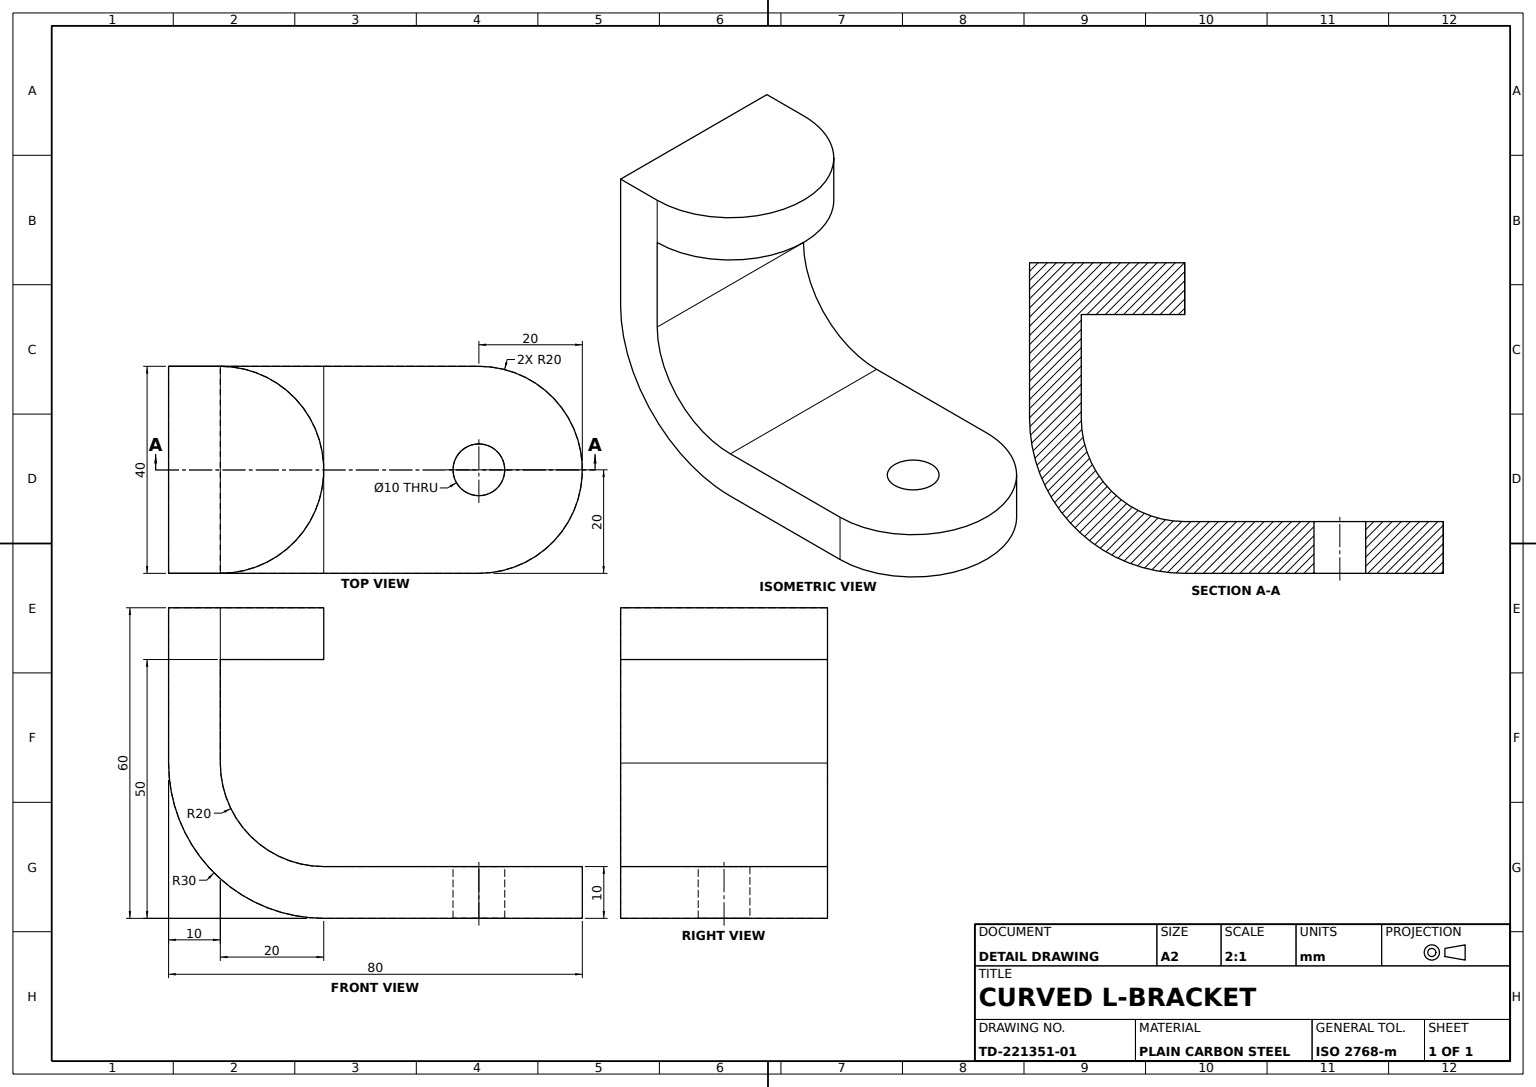
from build123d import *

# Parameters (mm, degrees)
CURVED_BRACKET_WALL_DEPTH = 40
ROUNDED_END_TAB_DEPTH     = 10
MOUNTING_TAB_DEPTH        = 10
MOUNTING_HOLE_SKETCH_R    = 5
MOUNTING_HOLE_10_DEPTH    = 10


with BuildPart() as part:
    # Bracket Profile Sketch → Curved Bracket Wall (new body)
    with BuildSketch(Plane.XY):
        with BuildLine():
            Line((50, 0), (20, 0))
            ThreePointArc((20, 0), (5.857864376, 5.857864376), (0, 20))
            Line((0, 20), (0, 50))
            Line((0, 50), (-10, 50))
            Line((-10, 50), (-10, 20))
            ThreePointArc((-10, 20), (-1.213203436, -1.213203436), (20, -10))
            Line((20, -10), (50, -10))
            Line((50, -10), (50, 0))
        make_face()
    extrude(amount=CURVED_BRACKET_WALL_DEPTH)

    # Rounded Tab Sketch → Rounded End Tab (add)
    with BuildSketch(Plane(origin=(0, 50, 0), x_dir=(1, 0, 0), z_dir=(0, 1, 0))):
        with BuildLine():
            Line((0, 0), (0, -40))
            ThreePointArc((0, -40), (20, -20), (0, 0))
        make_face()
    extrude(amount=-ROUNDED_END_TAB_DEPTH)

    # Mounting Tab Sketch → Mounting Tab (add)
    with BuildSketch(Plane(origin=(0, 0, 0), x_dir=(1, 0, 0), z_dir=(0, 1, 0))):
        with BuildLine():
            Line((50, 0), (50, -40))
            ThreePointArc((50, -40), (70, -20), (50, 0))
        make_face()
    extrude(amount=-MOUNTING_TAB_DEPTH)

    # Mounting Hole Sketch → Mounting Hole Ø10 (cut)
    with BuildSketch(Plane(origin=(0, 0, 0), x_dir=(1, 0, 0), z_dir=(0, 1, 0))):
        with Locations(Location((50, -20, 0), (0, 0, 270))):
            Circle(MOUNTING_HOLE_SKETCH_R)
    extrude(amount=-MOUNTING_HOLE_10_DEPTH, mode=Mode.SUBTRACT)


solid = part.part
